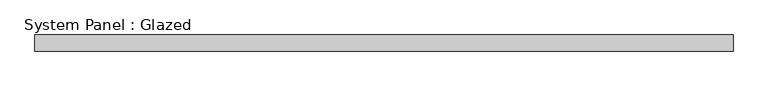
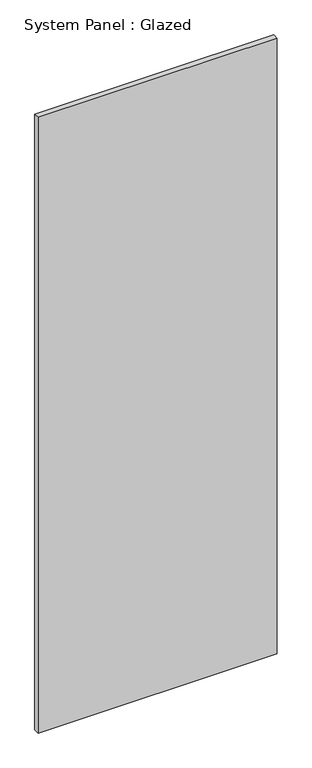
"""IFC4 building model written with IfcOpenShell, lengths in millimetres: plate geometry, System Panel : Glazed."""

from ifc_helpers import new_model, si_unit, origin, origin_with_axes, place, context, project, spatial, polyline, outline, extrude, source, transform, mapped, element, save


def system_panel_glazed_38c921e2(model_context):
    return source(origin(), model_context, "Body", "SweptSolid", [
        extrude(outline(polyline([(536.575, 19.05), (-536.575, 19.05), (-536.575, 44.45), (536.575, 44.45), (536.575, 19.05)])), origin_with_axes(), (0.0, 0.0, 1.0), 2921.0),
    ])


if __name__ == "__main__":
    model = new_model("IFC4")
    model_context = context("Model", 3, world=origin())
    ifc_project = project(units=[si_unit("LENGTHUNIT", "METRE", prefix="MILLI")], contexts=[model_context])
    site = spatial("IfcSite", under=ifc_project)
    building = spatial("IfcBuilding", under=site)
    placement = place(None, origin())
    system_panel_glazed_shape = system_panel_glazed_38c921e2(model_context)
    element("IfcPlate", 1, ObjectType="System Panel : Glazed", at=placement, inside=building, context=model_context, shape_type="MappedRepresentation", body=[
        mapped(system_panel_glazed_shape, transform((0.0, 0.0, 0.0), x_axis=(1.0, 0.0, 0.0), y_axis=(0.0, 1.0, 0.0), z_axis=(0.0, 0.0, 1.0))),
    ])
    save(model, "model.ifc")

# Revit data of these elements
# Type "System Panel : Glazed"
#   Construction Type Id = "GSP4R"
#   Analytic Construction = "1/8 in Pilkington single glazing"
#   Visual Light Transmittance = 0.9
#   Solar Heat Gain Coefficient = 0.86
#   Heat Transfer Coefficient (U) = 1.18115 BTU/(h·ft²·°F)
# Element 1 (IfcPlate, "System Panel : Glazed")
#   Materials on its faces: "Glass"
# Materials
#   "Glass": class "Glass", colour RGB 0 128 192, transparency 0.75, Description = "Soda Lime Glass", Cost = 0
